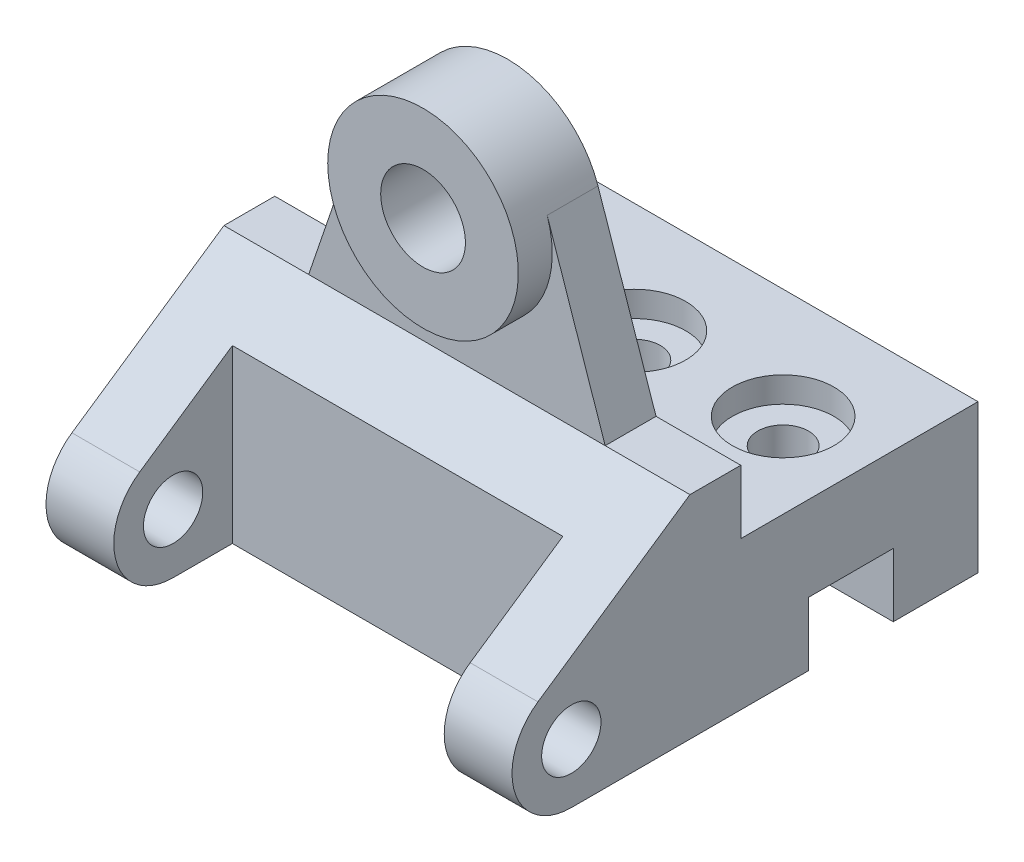
ISO-10303-21;
HEADER;
FILE_DESCRIPTION(('STEP AP214'),'2;1');
FILE_NAME('part.step','',(''),(''),'','','');
FILE_SCHEMA(('AUTOMOTIVE_DESIGN { 1 0 10303 214 1 1 1 1 }'));
ENDSEC;
DATA;
#1=APPLICATION_CONTEXT('core data for automotive mechanical design processes');
#2=APPLICATION_PROTOCOL_DEFINITION('international standard','automotive_design',2000,#1);
#3=PRODUCT_CONTEXT('',#1,'mechanical');
#4=PRODUCT('Part','Part','',(#3));
#5=PRODUCT_RELATED_PRODUCT_CATEGORY('part','',(#4));
#6=PRODUCT_DEFINITION_FORMATION('','',#4);
#7=PRODUCT_DEFINITION_CONTEXT('part definition',#1,'design');
#8=PRODUCT_DEFINITION('design','',#6,#7);
#9=PRODUCT_DEFINITION_SHAPE('','',#8);
#10=(LENGTH_UNIT() NAMED_UNIT(*) SI_UNIT(.MILLI.,.METRE.));
#11=(NAMED_UNIT(*) PLANE_ANGLE_UNIT() SI_UNIT($,.RADIAN.));
#12=(NAMED_UNIT(*) SI_UNIT($,.STERADIAN.) SOLID_ANGLE_UNIT());
#13=UNCERTAINTY_MEASURE_WITH_UNIT(LENGTH_MEASURE(1.E-05),#10,'distance_accuracy_value','');
#14=(GEOMETRIC_REPRESENTATION_CONTEXT(3) GLOBAL_UNCERTAINTY_ASSIGNED_CONTEXT((#13)) GLOBAL_UNIT_ASSIGNED_CONTEXT((#10,
#11,#12)) REPRESENTATION_CONTEXT('',''));
#15=CARTESIAN_POINT('',(0.,0.,0.));
#16=DIRECTION('',(0.,0.,1.));
#17=DIRECTION('',(1.,0.,0.));
#18=AXIS2_PLACEMENT_3D('',#15,#16,#17);
#19=CARTESIAN_POINT('',(55.,50.,28.));
#20=DIRECTION('',(0.,-1.,0.));
#21=DIRECTION('',(0.,0.,-1.));
#22=AXIS2_PLACEMENT_3D('',#19,#20,#21);
#23=PLANE('',#22);
#24=DIRECTION('',(0.,0.,-1.));
#25=VECTOR('',#24,1.);
#26=CARTESIAN_POINT('',(35.,50.,28.));
#27=LINE('',#26,#25);
#28=CARTESIAN_POINT('',(35.,50.,28.));
#29=VERTEX_POINT('',#28);
#30=CARTESIAN_POINT('',(35.,50.,16.));
#31=VERTEX_POINT('',#30);
#32=EDGE_CURVE('E224',#29,#31,#27,.T.);
#33=ORIENTED_EDGE('',*,*,#32,.F.);
#34=DIRECTION('',(-1.,0.,0.));
#35=VECTOR('',#34,1.);
#36=CARTESIAN_POINT('',(55.,50.,28.));
#37=LINE('',#36,#35);
#38=CARTESIAN_POINT('',(55.,50.,28.));
#39=VERTEX_POINT('',#38);
#40=EDGE_CURVE('E401',#39,#29,#37,.T.);
#41=ORIENTED_EDGE('',*,*,#40,.F.);
#42=DIRECTION('',(0.,0.,1.));
#43=VECTOR('',#42,1.);
#44=CARTESIAN_POINT('',(55.,50.,28.));
#45=LINE('',#44,#43);
#46=CARTESIAN_POINT('',(55.,50.,16.));
#47=VERTEX_POINT('',#46);
#48=EDGE_CURVE('E269',#47,#39,#45,.T.);
#49=ORIENTED_EDGE('',*,*,#48,.F.);
#50=DIRECTION('',(-1.,0.,0.));
#51=VECTOR('',#50,1.);
#52=CARTESIAN_POINT('',(55.,50.,16.));
#53=LINE('',#52,#51);
#54=EDGE_CURVE('E408',#47,#31,#53,.T.);
#55=ORIENTED_EDGE('',*,*,#54,.T.);
#56=EDGE_LOOP('',(#33,#41,#49,#55));
#57=FACE_BOUND('',#56,.T.);
#58=ADVANCED_FACE('F43',(#57),#23,.F.);
#59=CARTESIAN_POINT('',(55.,25.5724937407409,63.8789205238098));
#60=DIRECTION('',(0.,-0.826606695767211,-0.562780037414986));
#61=DIRECTION('',(0.,0.562780037414986,-0.826606695767211));
#62=AXIS2_PLACEMENT_3D('',#59,#60,#61);
#63=PLANE('',#62);
#64=DIRECTION('',(0.,-0.562780037414986,0.826606695767211));
#65=VECTOR('',#64,1.);
#66=CARTESIAN_POINT('',(-39.,25.5724937407409,63.8789205238098));
#67=LINE('',#66,#65);
#68=CARTESIAN_POINT('',(-39.,40.4683562761405,42.));
#69=VERTEX_POINT('',#68);
#70=CARTESIAN_POINT('',(-39.,25.5724937407409,63.8789205238098));
#71=VERTEX_POINT('',#70);
#72=EDGE_CURVE('E251',#69,#71,#67,.T.);
#73=ORIENTED_EDGE('',*,*,#72,.F.);
#74=DIRECTION('',(1.,0.,0.));
#75=VECTOR('',#74,1.);
#76=CARTESIAN_POINT('',(-39.,40.4683562761405,42.));
#77=LINE('',#76,#75);
#78=CARTESIAN_POINT('',(39.,40.4683562761405,42.));
#79=VERTEX_POINT('',#78);
#80=EDGE_CURVE('E238',#69,#79,#77,.T.);
#81=ORIENTED_EDGE('',*,*,#80,.T.);
#82=DIRECTION('',(0.,-0.562780037414986,0.826606695767211));
#83=VECTOR('',#82,1.);
#84=CARTESIAN_POINT('',(39.,25.5724937407409,63.8789205238098));
#85=LINE('',#84,#83);
#86=CARTESIAN_POINT('',(39.,25.5724937407409,63.8789205238098));
#87=VERTEX_POINT('',#86);
#88=EDGE_CURVE('E246',#79,#87,#85,.T.);
#89=ORIENTED_EDGE('',*,*,#88,.T.);
#90=DIRECTION('',(-1.,0.,0.));
#91=VECTOR('',#90,1.);
#92=CARTESIAN_POINT('',(55.,25.5724937407409,63.8789205238098));
#93=LINE('',#92,#91);
#94=CARTESIAN_POINT('',(55.,25.5724937407409,63.8789205238098));
#95=VERTEX_POINT('',#94);
#96=EDGE_CURVE('E412',#95,#87,#93,.T.);
#97=ORIENTED_EDGE('',*,*,#96,.F.);
#98=DIRECTION('',(0.,-0.562780037414986,0.826606695767211));
#99=VECTOR('',#98,1.);
#100=CARTESIAN_POINT('',(55.,25.5724937407409,63.8789205238098));
#101=LINE('',#100,#99);
#102=EDGE_CURVE('E275',#39,#95,#101,.T.);
#103=ORIENTED_EDGE('',*,*,#102,.F.);
#104=ORIENTED_EDGE('',*,*,#40,.T.);
#105=DIRECTION('',(1.,0.,0.));
#106=VECTOR('',#105,1.);
#107=CARTESIAN_POINT('',(0.,50.,28.));
#108=LINE('',#107,#106);
#109=CARTESIAN_POINT('',(-35.,50.,28.));
#110=VERTEX_POINT('',#109);
#111=EDGE_CURVE('E214',#110,#29,#108,.T.);
#112=ORIENTED_EDGE('',*,*,#111,.F.);
#113=CARTESIAN_POINT('',(-55.,50.,28.));
#114=VERTEX_POINT('',#113);
#115=EDGE_CURVE('E411',#110,#114,#37,.T.);
#116=ORIENTED_EDGE('',*,*,#115,.T.);
#117=DIRECTION('',(0.,-0.562780037414986,0.826606695767211));
#118=VECTOR('',#117,1.);
#119=CARTESIAN_POINT('',(-55.,25.5724937407409,63.8789205238098));
#120=LINE('',#119,#118);
#121=CARTESIAN_POINT('',(-55.,25.5724937407409,63.8789205238098));
#122=VERTEX_POINT('',#121);
#123=EDGE_CURVE('E298',#114,#122,#120,.T.);
#124=ORIENTED_EDGE('',*,*,#123,.T.);
#125=EDGE_CURVE('E438',#71,#122,#93,.T.);
#126=ORIENTED_EDGE('',*,*,#125,.F.);
#127=EDGE_LOOP('',(#73,#81,#89,#97,#103,#104,#112,#116,#124,#126));
#128=FACE_BOUND('',#127,.T.);
#129=ADVANCED_FACE('F409',(#128),#63,.F.);
#130=CARTESIAN_POINT('',(55.,14.,56.));
#131=DIRECTION('',(-1.,0.,0.));
#132=DIRECTION('',(0.,0.,1.));
#133=AXIS2_PLACEMENT_3D('',#130,#131,#132);
#134=CYLINDRICAL_SURFACE('',#133,14.);
#135=CARTESIAN_POINT('',(-39.,14.,56.));
#136=DIRECTION('',(1.,0.,0.));
#137=DIRECTION('',(0.,0.,-1.));
#138=AXIS2_PLACEMENT_3D('',#135,#136,#137);
#139=CIRCLE('',#138,14.);
#140=CARTESIAN_POINT('',(-39.,0.,56.));
#141=VERTEX_POINT('',#140);
#142=EDGE_CURVE('E253',#71,#141,#139,.T.);
#143=ORIENTED_EDGE('',*,*,#142,.F.);
#144=ORIENTED_EDGE('',*,*,#125,.T.);
#145=CARTESIAN_POINT('',(-55.,14.,56.));
#146=DIRECTION('',(1.,0.,0.));
#147=DIRECTION('',(0.,0.,1.));
#148=AXIS2_PLACEMENT_3D('',#145,#146,#147);
#149=CIRCLE('',#148,14.);
#150=CARTESIAN_POINT('',(-55.,0.,56.));
#151=VERTEX_POINT('',#150);
#152=EDGE_CURVE('E297',#122,#151,#149,.T.);
#153=ORIENTED_EDGE('',*,*,#152,.T.);
#154=DIRECTION('',(-1.,0.,0.));
#155=VECTOR('',#154,1.);
#156=CARTESIAN_POINT('',(55.,0.,56.));
#157=LINE('',#156,#155);
#158=EDGE_CURVE('E439',#141,#151,#157,.T.);
#159=ORIENTED_EDGE('',*,*,#158,.F.);
#160=EDGE_LOOP('',(#143,#144,#153,#159));
#161=FACE_BOUND('',#160,.T.);
#162=ADVANCED_FACE('F437',(#161),#134,.T.);
#163=CARTESIAN_POINT('',(55.,14.,56.));
#164=DIRECTION('',(-1.,0.,0.));
#165=DIRECTION('',(0.,0.,1.));
#166=AXIS2_PLACEMENT_3D('',#163,#164,#165);
#167=CYLINDRICAL_SURFACE('',#166,7.);
#168=CARTESIAN_POINT('',(-55.,14.,56.));
#169=DIRECTION('',(1.,0.,0.));
#170=DIRECTION('',(0.,0.,-1.));
#171=AXIS2_PLACEMENT_3D('',#168,#169,#170);
#172=CIRCLE('',#171,7.);
#173=CARTESIAN_POINT('',(-55.,14.,49.));
#174=VERTEX_POINT('',#173);
#175=EDGE_CURVE('E254',#174,#174,#172,.T.);
#176=ORIENTED_EDGE('',*,*,#175,.F.);
#177=EDGE_LOOP('',(#176));
#178=FACE_BOUND('',#177,.T.);
#179=CARTESIAN_POINT('',(-39.,14.,56.));
#180=DIRECTION('',(1.,0.,0.));
#181=DIRECTION('',(0.,0.,-1.));
#182=AXIS2_PLACEMENT_3D('',#179,#180,#181);
#183=CIRCLE('',#182,7.);
#184=CARTESIAN_POINT('',(-39.,14.,49.));
#185=VERTEX_POINT('',#184);
#186=EDGE_CURVE('E247',#185,#185,#183,.T.);
#187=ORIENTED_EDGE('',*,*,#186,.T.);
#188=EDGE_LOOP('',(#187));
#189=FACE_BOUND('',#188,.T.);
#190=ADVANCED_FACE('F422',(#178,#189),#167,.F.);
#191=CARTESIAN_POINT('',(55.,14.,56.));
#192=DIRECTION('',(-1.,0.,0.));
#193=DIRECTION('',(0.,0.,1.));
#194=AXIS2_PLACEMENT_3D('',#191,#192,#193);
#195=PLANE('',#194);
#196=DIRECTION('',(0.,1.,0.));
#197=VECTOR('',#196,1.);
#198=CARTESIAN_POINT('',(55.,35.,-40.));
#199=LINE('',#198,#197);
#200=CARTESIAN_POINT('',(55.,0.,-40.));
#201=VERTEX_POINT('',#200);
#202=CARTESIAN_POINT('',(55.,35.,-40.));
#203=VERTEX_POINT('',#202);
#204=EDGE_CURVE('E265',#201,#203,#199,.T.);
#205=ORIENTED_EDGE('',*,*,#204,.T.);
#206=DIRECTION('',(0.,0.,1.));
#207=VECTOR('',#206,1.);
#208=CARTESIAN_POINT('',(55.,35.,16.));
#209=LINE('',#208,#207);
#210=CARTESIAN_POINT('',(55.,35.,16.));
#211=VERTEX_POINT('',#210);
#212=EDGE_CURVE('E264',#203,#211,#209,.T.);
#213=ORIENTED_EDGE('',*,*,#212,.T.);
#214=DIRECTION('',(0.,1.,0.));
#215=VECTOR('',#214,1.);
#216=CARTESIAN_POINT('',(55.,50.,16.));
#217=LINE('',#216,#215);
#218=EDGE_CURVE('E268',#211,#47,#217,.T.);
#219=ORIENTED_EDGE('',*,*,#218,.T.);
#220=ORIENTED_EDGE('',*,*,#48,.T.);
#221=ORIENTED_EDGE('',*,*,#102,.T.);
#222=CARTESIAN_POINT('',(55.,14.,56.));
#223=DIRECTION('',(1.,0.,0.));
#224=DIRECTION('',(0.,0.,1.));
#225=AXIS2_PLACEMENT_3D('',#222,#223,#224);
#226=CIRCLE('',#225,14.);
#227=CARTESIAN_POINT('',(55.,0.,56.));
#228=VERTEX_POINT('',#227);
#229=EDGE_CURVE('E273',#95,#228,#226,.T.);
#230=ORIENTED_EDGE('',*,*,#229,.T.);
#231=DIRECTION('',(0.,0.,-1.));
#232=VECTOR('',#231,1.);
#233=CARTESIAN_POINT('',(55.,0.,0.));
#234=LINE('',#233,#232);
#235=CARTESIAN_POINT('',(55.,0.,0.));
#236=VERTEX_POINT('',#235);
#237=EDGE_CURVE('E277',#228,#236,#234,.T.);
#238=ORIENTED_EDGE('',*,*,#237,.T.);
#239=DIRECTION('',(0.,1.,0.));
#240=VECTOR('',#239,1.);
#241=CARTESIAN_POINT('',(55.,0.,0.));
#242=LINE('',#241,#240);
#243=CARTESIAN_POINT('',(55.,15.,0.));
#244=VERTEX_POINT('',#243);
#245=EDGE_CURVE('E279',#236,#244,#242,.T.);
#246=ORIENTED_EDGE('',*,*,#245,.T.);
#247=DIRECTION('',(0.,0.,-1.));
#248=VECTOR('',#247,1.);
#249=CARTESIAN_POINT('',(55.,15.,0.));
#250=LINE('',#249,#248);
#251=CARTESIAN_POINT('',(55.,15.,-20.));
#252=VERTEX_POINT('',#251);
#253=EDGE_CURVE('E278',#244,#252,#250,.T.);
#254=ORIENTED_EDGE('',*,*,#253,.T.);
#255=DIRECTION('',(0.,-1.,0.));
#256=VECTOR('',#255,1.);
#257=CARTESIAN_POINT('',(55.,0.,-20.));
#258=LINE('',#257,#256);
#259=CARTESIAN_POINT('',(55.,0.,-20.));
#260=VERTEX_POINT('',#259);
#261=EDGE_CURVE('E285',#252,#260,#258,.T.);
#262=ORIENTED_EDGE('',*,*,#261,.T.);
#263=DIRECTION('',(0.,0.,-1.));
#264=VECTOR('',#263,1.);
#265=CARTESIAN_POINT('',(55.,0.,-40.));
#266=LINE('',#265,#264);
#267=EDGE_CURVE('E282',#260,#201,#266,.T.);
#268=ORIENTED_EDGE('',*,*,#267,.T.);
#269=EDGE_LOOP('',(#205,#213,#219,#220,#221,#230,#238,#246,#254,#262,#268));
#270=FACE_BOUND('',#269,.T.);
#271=CARTESIAN_POINT('',(55.,14.,56.));
#272=DIRECTION('',(1.,0.,0.));
#273=DIRECTION('',(0.,0.,-1.));
#274=AXIS2_PLACEMENT_3D('',#271,#272,#273);
#275=CIRCLE('',#274,7.);
#276=CARTESIAN_POINT('',(55.,14.,49.));
#277=VERTEX_POINT('',#276);
#278=EDGE_CURVE('E258',#277,#277,#275,.T.);
#279=ORIENTED_EDGE('',*,*,#278,.F.);
#280=EDGE_LOOP('',(#279));
#281=FACE_BOUND('',#280,.T.);
#282=ADVANCED_FACE('F359',(#270,#281),#195,.F.);
#283=CARTESIAN_POINT('',(-55.,14.,56.));
#284=DIRECTION('',(-1.,0.,0.));
#285=DIRECTION('',(0.,0.,1.));
#286=AXIS2_PLACEMENT_3D('',#283,#284,#285);
#287=PLANE('',#286);
#288=DIRECTION('',(0.,1.,0.));
#289=VECTOR('',#288,1.);
#290=CARTESIAN_POINT('',(-55.,35.,-40.));
#291=LINE('',#290,#289);
#292=CARTESIAN_POINT('',(-55.,0.,-40.));
#293=VERTEX_POINT('',#292);
#294=CARTESIAN_POINT('',(-55.,35.,-40.));
#295=VERTEX_POINT('',#294);
#296=EDGE_CURVE('E259',#293,#295,#291,.T.);
#297=ORIENTED_EDGE('',*,*,#296,.F.);
#298=DIRECTION('',(0.,0.,-1.));
#299=VECTOR('',#298,1.);
#300=CARTESIAN_POINT('',(-55.,0.,-40.));
#301=LINE('',#300,#299);
#302=CARTESIAN_POINT('',(-55.,0.,-20.));
#303=VERTEX_POINT('',#302);
#304=EDGE_CURVE('E266',#303,#293,#301,.T.);
#305=ORIENTED_EDGE('',*,*,#304,.F.);
#306=DIRECTION('',(0.,-1.,0.));
#307=VECTOR('',#306,1.);
#308=CARTESIAN_POINT('',(-55.,0.,-20.));
#309=LINE('',#308,#307);
#310=CARTESIAN_POINT('',(-55.,15.,-20.));
#311=VERTEX_POINT('',#310);
#312=EDGE_CURVE('E310',#311,#303,#309,.T.);
#313=ORIENTED_EDGE('',*,*,#312,.F.);
#314=DIRECTION('',(0.,0.,-1.));
#315=VECTOR('',#314,1.);
#316=CARTESIAN_POINT('',(-55.,15.,0.));
#317=LINE('',#316,#315);
#318=CARTESIAN_POINT('',(-55.,15.,0.));
#319=VERTEX_POINT('',#318);
#320=EDGE_CURVE('E308',#319,#311,#317,.T.);
#321=ORIENTED_EDGE('',*,*,#320,.F.);
#322=DIRECTION('',(0.,1.,0.));
#323=VECTOR('',#322,1.);
#324=CARTESIAN_POINT('',(-55.,0.,0.));
#325=LINE('',#324,#323);
#326=CARTESIAN_POINT('',(-55.,0.,0.));
#327=VERTEX_POINT('',#326);
#328=EDGE_CURVE('E303',#327,#319,#325,.T.);
#329=ORIENTED_EDGE('',*,*,#328,.F.);
#330=DIRECTION('',(0.,0.,-1.));
#331=VECTOR('',#330,1.);
#332=CARTESIAN_POINT('',(-55.,0.,0.));
#333=LINE('',#332,#331);
#334=EDGE_CURVE('E301',#151,#327,#333,.T.);
#335=ORIENTED_EDGE('',*,*,#334,.F.);
#336=ORIENTED_EDGE('',*,*,#152,.F.);
#337=ORIENTED_EDGE('',*,*,#123,.F.);
#338=DIRECTION('',(0.,0.,1.));
#339=VECTOR('',#338,1.);
#340=CARTESIAN_POINT('',(-55.,50.,28.));
#341=LINE('',#340,#339);
#342=CARTESIAN_POINT('',(-55.,50.,16.));
#343=VERTEX_POINT('',#342);
#344=EDGE_CURVE('E291',#343,#114,#341,.T.);
#345=ORIENTED_EDGE('',*,*,#344,.F.);
#346=DIRECTION('',(0.,1.,0.));
#347=VECTOR('',#346,1.);
#348=CARTESIAN_POINT('',(-55.,50.,16.));
#349=LINE('',#348,#347);
#350=CARTESIAN_POINT('',(-55.,35.,16.));
#351=VERTEX_POINT('',#350);
#352=EDGE_CURVE('E292',#351,#343,#349,.T.);
#353=ORIENTED_EDGE('',*,*,#352,.F.);
#354=DIRECTION('',(0.,0.,1.));
#355=VECTOR('',#354,1.);
#356=CARTESIAN_POINT('',(-55.,35.,16.));
#357=LINE('',#356,#355);
#358=EDGE_CURVE('E288',#295,#351,#357,.T.);
#359=ORIENTED_EDGE('',*,*,#358,.F.);
#360=EDGE_LOOP('',(#297,#305,#313,#321,#329,#335,#336,#337,#345,#353,#359));
#361=FACE_BOUND('',#360,.T.);
#362=ORIENTED_EDGE('',*,*,#175,.T.);
#363=EDGE_LOOP('',(#362));
#364=FACE_BOUND('',#363,.T.);
#365=ADVANCED_FACE('F347',(#361,#364),#287,.T.);
#366=CARTESIAN_POINT('',(55.,35.,-40.));
#367=DIRECTION('',(0.,0.,1.));
#368=DIRECTION('',(0.,-1.,0.));
#369=AXIS2_PLACEMENT_3D('',#366,#367,#368);
#370=PLANE('',#369);
#371=ORIENTED_EDGE('',*,*,#296,.T.);
#372=DIRECTION('',(-1.,0.,0.));
#373=VECTOR('',#372,1.);
#374=CARTESIAN_POINT('',(55.,35.,-40.));
#375=LINE('',#374,#373);
#376=EDGE_CURVE('E12',#203,#295,#375,.T.);
#377=ORIENTED_EDGE('',*,*,#376,.F.);
#378=ORIENTED_EDGE('',*,*,#204,.F.);
#379=DIRECTION('',(-1.,0.,0.));
#380=VECTOR('',#379,1.);
#381=CARTESIAN_POINT('',(55.,0.,-40.));
#382=LINE('',#381,#380);
#383=EDGE_CURVE('E289',#201,#293,#382,.T.);
#384=ORIENTED_EDGE('',*,*,#383,.T.);
#385=EDGE_LOOP('',(#371,#377,#378,#384));
#386=FACE_BOUND('',#385,.T.);
#387=ADVANCED_FACE('F44',(#386),#370,.F.);
#388=CARTESIAN_POINT('',(55.,35.,16.));
#389=DIRECTION('',(0.,-1.,0.));
#390=DIRECTION('',(0.,0.,-1.));
#391=AXIS2_PLACEMENT_3D('',#388,#389,#390);
#392=PLANE('',#391);
#393=CARTESIAN_POINT('',(35.,35.,-14.));
#394=DIRECTION('',(0.,1.,0.));
#395=DIRECTION('',(0.,0.,1.));
#396=AXIS2_PLACEMENT_3D('',#393,#394,#395);
#397=CIRCLE('',#396,12.);
#398=CARTESIAN_POINT('',(35.,35.,-1.99999999999999));
#399=VERTEX_POINT('',#398);
#400=EDGE_CURVE('E575',#399,#399,#397,.T.);
#401=ORIENTED_EDGE('',*,*,#400,.F.);
#402=EDGE_LOOP('',(#401));
#403=FACE_BOUND('',#402,.T.);
#404=CARTESIAN_POINT('',(0.,35.,-14.));
#405=DIRECTION('',(0.,1.,0.));
#406=DIRECTION('',(0.,0.,1.));
#407=AXIS2_PLACEMENT_3D('',#404,#405,#406);
#408=CIRCLE('',#407,12.);
#409=CARTESIAN_POINT('',(0.,35.,-1.99999999999999));
#410=VERTEX_POINT('',#409);
#411=EDGE_CURVE('E583',#410,#410,#408,.T.);
#412=ORIENTED_EDGE('',*,*,#411,.F.);
#413=EDGE_LOOP('',(#412));
#414=FACE_BOUND('',#413,.T.);
#415=CARTESIAN_POINT('',(-35.,35.,-14.));
#416=DIRECTION('',(0.,1.,0.));
#417=DIRECTION('',(0.,0.,1.));
#418=AXIS2_PLACEMENT_3D('',#415,#416,#417);
#419=CIRCLE('',#418,12.);
#420=CARTESIAN_POINT('',(-35.,35.,-1.99999999999999));
#421=VERTEX_POINT('',#420);
#422=EDGE_CURVE('E365',#421,#421,#419,.T.);
#423=ORIENTED_EDGE('',*,*,#422,.F.);
#424=EDGE_LOOP('',(#423));
#425=FACE_BOUND('',#424,.T.);
#426=ORIENTED_EDGE('',*,*,#358,.T.);
#427=DIRECTION('',(-1.,0.,0.));
#428=VECTOR('',#427,1.);
#429=CARTESIAN_POINT('',(55.,35.,16.));
#430=LINE('',#429,#428);
#431=EDGE_CURVE('E52',#211,#351,#430,.T.);
#432=ORIENTED_EDGE('',*,*,#431,.F.);
#433=ORIENTED_EDGE('',*,*,#212,.F.);
#434=ORIENTED_EDGE('',*,*,#376,.T.);
#435=EDGE_LOOP('',(#426,#432,#433,#434));
#436=FACE_BOUND('',#435,.T.);
#437=ADVANCED_FACE('F481',(#403,#414,#425,#436),#392,.F.);
#438=CARTESIAN_POINT('',(55.,50.,16.));
#439=DIRECTION('',(0.,0.,1.));
#440=DIRECTION('',(0.,-1.,0.));
#441=AXIS2_PLACEMENT_3D('',#438,#439,#440);
#442=PLANE('',#441);
#443=ORIENTED_EDGE('',*,*,#352,.T.);
#444=CARTESIAN_POINT('',(-35.,50.,16.));
#445=VERTEX_POINT('',#444);
#446=EDGE_CURVE('E211',#445,#343,#53,.T.);
#447=ORIENTED_EDGE('',*,*,#446,.F.);
#448=DIRECTION('',(-0.322220189663275,-0.946664750253945,0.));
#449=VECTOR('',#448,1.);
#450=CARTESIAN_POINT('',(-46.6178199967859,15.8674998694345,16.));
#451=LINE('',#450,#449);
#452=CARTESIAN_POINT('',(-21.2999568807138,90.2499542674237,16.));
#453=VERTEX_POINT('',#452);
#454=EDGE_CURVE('E205',#453,#445,#451,.T.);
#455=ORIENTED_EDGE('',*,*,#454,.F.);
#456=CARTESIAN_POINT('',(0.,83.,16.));
#457=DIRECTION('',(0.,0.,-1.));
#458=DIRECTION('',(-1.,0.,0.));
#459=AXIS2_PLACEMENT_3D('',#456,#457,#458);
#460=CIRCLE('',#459,22.5);
#461=CARTESIAN_POINT('',(21.2999568807138,90.2499542674237,16.));
#462=VERTEX_POINT('',#461);
#463=EDGE_CURVE('E184',#453,#462,#460,.T.);
#464=ORIENTED_EDGE('',*,*,#463,.T.);
#465=DIRECTION('',(0.322220189663275,-0.946664750253945,0.));
#466=VECTOR('',#465,1.);
#467=CARTESIAN_POINT('',(46.6178199967858,15.8674998694345,16.));
#468=LINE('',#467,#466);
#469=EDGE_CURVE('E215',#462,#31,#468,.T.);
#470=ORIENTED_EDGE('',*,*,#469,.T.);
#471=ORIENTED_EDGE('',*,*,#54,.F.);
#472=ORIENTED_EDGE('',*,*,#218,.F.);
#473=ORIENTED_EDGE('',*,*,#431,.T.);
#474=EDGE_LOOP('',(#443,#447,#455,#464,#470,#471,#472,#473));
#475=FACE_BOUND('',#474,.T.);
#476=CARTESIAN_POINT('',(0.,83.,16.));
#477=DIRECTION('',(0.,0.,-1.));
#478=DIRECTION('',(-1.,0.,0.));
#479=AXIS2_PLACEMENT_3D('',#476,#477,#478);
#480=CIRCLE('',#479,10.);
#481=CARTESIAN_POINT('',(-10.,83.,16.));
#482=VERTEX_POINT('',#481);
#483=EDGE_CURVE('E198',#482,#482,#480,.T.);
#484=ORIENTED_EDGE('',*,*,#483,.F.);
#485=EDGE_LOOP('',(#484));
#486=FACE_BOUND('',#485,.T.);
#487=ADVANCED_FACE('F207',(#475,#486),#442,.F.);
#488=ORIENTED_EDGE('',*,*,#115,.F.);
#489=DIRECTION('',(0.,0.,-1.));
#490=VECTOR('',#489,1.);
#491=CARTESIAN_POINT('',(-35.,50.,28.));
#492=LINE('',#491,#490);
#493=EDGE_CURVE('E202',#110,#445,#492,.T.);
#494=ORIENTED_EDGE('',*,*,#493,.T.);
#495=ORIENTED_EDGE('',*,*,#446,.T.);
#496=ORIENTED_EDGE('',*,*,#344,.T.);
#497=EDGE_LOOP('',(#488,#494,#495,#496));
#498=FACE_BOUND('',#497,.T.);
#499=ADVANCED_FACE('F472',(#498),#23,.F.);
#500=ORIENTED_EDGE('',*,*,#96,.T.);
#501=CARTESIAN_POINT('',(39.,14.,56.));
#502=DIRECTION('',(1.,0.,0.));
#503=DIRECTION('',(0.,0.,-1.));
#504=AXIS2_PLACEMENT_3D('',#501,#502,#503);
#505=CIRCLE('',#504,14.);
#506=CARTESIAN_POINT('',(39.,0.,56.));
#507=VERTEX_POINT('',#506);
#508=EDGE_CURVE('E244',#87,#507,#505,.T.);
#509=ORIENTED_EDGE('',*,*,#508,.T.);
#510=EDGE_CURVE('E444',#228,#507,#157,.T.);
#511=ORIENTED_EDGE('',*,*,#510,.F.);
#512=ORIENTED_EDGE('',*,*,#229,.F.);
#513=EDGE_LOOP('',(#500,#509,#511,#512));
#514=FACE_BOUND('',#513,.T.);
#515=ADVANCED_FACE('F464',(#514),#134,.T.);
#516=CARTESIAN_POINT('',(55.,0.,0.));
#517=DIRECTION('',(0.,1.,0.));
#518=DIRECTION('',(0.,0.,1.));
#519=AXIS2_PLACEMENT_3D('',#516,#517,#518);
#520=PLANE('',#519);
#521=ORIENTED_EDGE('',*,*,#510,.T.);
#522=DIRECTION('',(0.,0.,-1.));
#523=VECTOR('',#522,1.);
#524=CARTESIAN_POINT('',(39.,0.,70.));
#525=LINE('',#524,#523);
#526=CARTESIAN_POINT('',(39.,0.,42.));
#527=VERTEX_POINT('',#526);
#528=EDGE_CURVE('E223',#507,#527,#525,.T.);
#529=ORIENTED_EDGE('',*,*,#528,.T.);
#530=DIRECTION('',(1.,0.,0.));
#531=VECTOR('',#530,1.);
#532=CARTESIAN_POINT('',(-39.,0.,42.));
#533=LINE('',#532,#531);
#534=CARTESIAN_POINT('',(-39.,0.,42.));
#535=VERTEX_POINT('',#534);
#536=EDGE_CURVE('E232',#535,#527,#533,.T.);
#537=ORIENTED_EDGE('',*,*,#536,.F.);
#538=DIRECTION('',(0.,0.,-1.));
#539=VECTOR('',#538,1.);
#540=CARTESIAN_POINT('',(-39.,0.,70.));
#541=LINE('',#540,#539);
#542=EDGE_CURVE('E226',#141,#535,#541,.T.);
#543=ORIENTED_EDGE('',*,*,#542,.F.);
#544=ORIENTED_EDGE('',*,*,#158,.T.);
#545=ORIENTED_EDGE('',*,*,#334,.T.);
#546=DIRECTION('',(-1.,0.,0.));
#547=VECTOR('',#546,1.);
#548=CARTESIAN_POINT('',(55.,0.,0.));
#549=LINE('',#548,#547);
#550=EDGE_CURVE('E447',#236,#327,#549,.T.);
#551=ORIENTED_EDGE('',*,*,#550,.F.);
#552=ORIENTED_EDGE('',*,*,#237,.F.);
#553=EDGE_LOOP('',(#521,#529,#537,#543,#544,#545,#551,#552));
#554=FACE_BOUND('',#553,.T.);
#555=ADVANCED_FACE('F457',(#554),#520,.F.);
#556=CARTESIAN_POINT('',(55.,0.,0.));
#557=DIRECTION('',(0.,0.,1.));
#558=DIRECTION('',(0.,-1.,0.));
#559=AXIS2_PLACEMENT_3D('',#556,#557,#558);
#560=PLANE('',#559);
#561=ORIENTED_EDGE('',*,*,#328,.T.);
#562=DIRECTION('',(-1.,0.,0.));
#563=VECTOR('',#562,1.);
#564=CARTESIAN_POINT('',(55.,15.,0.));
#565=LINE('',#564,#563);
#566=EDGE_CURVE('E317',#244,#319,#565,.T.);
#567=ORIENTED_EDGE('',*,*,#566,.F.);
#568=ORIENTED_EDGE('',*,*,#245,.F.);
#569=ORIENTED_EDGE('',*,*,#550,.T.);
#570=EDGE_LOOP('',(#561,#567,#568,#569));
#571=FACE_BOUND('',#570,.T.);
#572=ADVANCED_FACE('F453',(#571),#560,.F.);
#573=CARTESIAN_POINT('',(55.,15.,0.));
#574=DIRECTION('',(0.,1.,0.));
#575=DIRECTION('',(0.,0.,1.));
#576=AXIS2_PLACEMENT_3D('',#573,#574,#575);
#577=PLANE('',#576);
#578=DIRECTION('',(-1.,0.,0.));
#579=VECTOR('',#578,1.);
#580=CARTESIAN_POINT('',(55.,15.,-20.));
#581=LINE('',#580,#579);
#582=CARTESIAN_POINT('',(35.,14.9995,-20.));
#583=VERTEX_POINT('',#582);
#584=CARTESIAN_POINT('',(0.,14.9995,-20.));
#585=VERTEX_POINT('',#584);
#586=EDGE_CURVE('E50',#583,#585,#581,.T.);
#587=ORIENTED_EDGE('',*,*,#586,.F.);
#588=CARTESIAN_POINT('',(35.,15.,-14.));
#589=DIRECTION('',(0.,1.,0.));
#590=DIRECTION('',(0.,0.,1.));
#591=AXIS2_PLACEMENT_3D('',#588,#589,#590);
#592=CIRCLE('',#591,6.00000000000001);
#593=EDGE_CURVE('E56',#583,#583,#592,.T.);
#594=ORIENTED_EDGE('',*,*,#593,.T.);
#595=EDGE_CURVE('E322',#252,#583,#581,.T.);
#596=ORIENTED_EDGE('',*,*,#595,.F.);
#597=ORIENTED_EDGE('',*,*,#253,.F.);
#598=ORIENTED_EDGE('',*,*,#566,.T.);
#599=ORIENTED_EDGE('',*,*,#320,.T.);
#600=CARTESIAN_POINT('',(-35.,14.9995,-20.));
#601=VERTEX_POINT('',#600);
#602=EDGE_CURVE('E316',#601,#311,#581,.T.);
#603=ORIENTED_EDGE('',*,*,#602,.F.);
#604=CARTESIAN_POINT('',(-35.,15.,-14.));
#605=DIRECTION('',(0.,1.,0.));
#606=DIRECTION('',(0.,0.,1.));
#607=AXIS2_PLACEMENT_3D('',#604,#605,#606);
#608=CIRCLE('',#607,6.00000000000001);
#609=EDGE_CURVE('E385',#601,#601,#608,.T.);
#610=ORIENTED_EDGE('',*,*,#609,.T.);
#611=EDGE_CURVE('E327',#585,#601,#581,.T.);
#612=ORIENTED_EDGE('',*,*,#611,.F.);
#613=CARTESIAN_POINT('',(0.,15.,-14.));
#614=DIRECTION('',(0.,1.,0.));
#615=DIRECTION('',(0.,0.,1.));
#616=AXIS2_PLACEMENT_3D('',#613,#614,#615);
#617=CIRCLE('',#616,6.00000000000001);
#618=EDGE_CURVE('E362',#585,#585,#617,.T.);
#619=ORIENTED_EDGE('',*,*,#618,.T.);
#620=EDGE_LOOP('',(#587,#594,#596,#597,#598,#599,#603,#610,#612,#619));
#621=FACE_BOUND('',#620,.T.);
#622=ADVANCED_FACE('F337',(#621),#577,.F.);
#623=CARTESIAN_POINT('',(55.,0.,-20.));
#624=DIRECTION('',(0.,0.,-1.));
#625=DIRECTION('',(0.,1.,0.));
#626=AXIS2_PLACEMENT_3D('',#623,#624,#625);
#627=PLANE('',#626);
#628=ORIENTED_EDGE('',*,*,#595,.T.);
#629=ORIENTED_EDGE('',*,*,#586,.T.);
#630=ORIENTED_EDGE('',*,*,#611,.T.);
#631=ORIENTED_EDGE('',*,*,#602,.T.);
#632=ORIENTED_EDGE('',*,*,#312,.T.);
#633=DIRECTION('',(-1.,0.,0.));
#634=VECTOR('',#633,1.);
#635=CARTESIAN_POINT('',(55.,0.,-20.));
#636=LINE('',#635,#634);
#637=EDGE_CURVE('E314',#260,#303,#636,.T.);
#638=ORIENTED_EDGE('',*,*,#637,.F.);
#639=ORIENTED_EDGE('',*,*,#261,.F.);
#640=EDGE_LOOP('',(#628,#629,#630,#631,#632,#638,#639));
#641=FACE_BOUND('',#640,.T.);
#642=ADVANCED_FACE('F335',(#641),#627,.F.);
#643=CARTESIAN_POINT('',(55.,0.,-40.));
#644=DIRECTION('',(0.,1.,0.));
#645=DIRECTION('',(0.,0.,1.));
#646=AXIS2_PLACEMENT_3D('',#643,#644,#645);
#647=PLANE('',#646);
#648=ORIENTED_EDGE('',*,*,#304,.T.);
#649=ORIENTED_EDGE('',*,*,#383,.F.);
#650=ORIENTED_EDGE('',*,*,#267,.F.);
#651=ORIENTED_EDGE('',*,*,#637,.T.);
#652=EDGE_LOOP('',(#648,#649,#650,#651));
#653=FACE_BOUND('',#652,.T.);
#654=ADVANCED_FACE('F348',(#653),#647,.F.);
#655=CARTESIAN_POINT('',(39.,14.,56.));
#656=DIRECTION('',(1.,0.,0.));
#657=DIRECTION('',(0.,0.,-1.));
#658=AXIS2_PLACEMENT_3D('',#655,#656,#657);
#659=CIRCLE('',#658,7.);
#660=CARTESIAN_POINT('',(39.,14.,49.));
#661=VERTEX_POINT('',#660);
#662=EDGE_CURVE('E241',#661,#661,#659,.T.);
#663=ORIENTED_EDGE('',*,*,#662,.F.);
#664=EDGE_LOOP('',(#663));
#665=FACE_BOUND('',#664,.T.);
#666=ORIENTED_EDGE('',*,*,#278,.T.);
#667=EDGE_LOOP('',(#666));
#668=FACE_BOUND('',#667,.T.);
#669=ADVANCED_FACE('F431',(#665,#668),#167,.F.);
#670=CARTESIAN_POINT('',(-39.,0.,0.));
#671=DIRECTION('',(1.,0.,0.));
#672=DIRECTION('',(0.,0.,-1.));
#673=AXIS2_PLACEMENT_3D('',#670,#671,#672);
#674=PLANE('',#673);
#675=ORIENTED_EDGE('',*,*,#186,.F.);
#676=EDGE_LOOP('',(#675));
#677=FACE_BOUND('',#676,.T.);
#678=ORIENTED_EDGE('',*,*,#72,.T.);
#679=ORIENTED_EDGE('',*,*,#142,.T.);
#680=ORIENTED_EDGE('',*,*,#542,.T.);
#681=DIRECTION('',(0.,1.,0.));
#682=VECTOR('',#681,1.);
#683=CARTESIAN_POINT('',(-39.,40.4683562761405,42.));
#684=LINE('',#683,#682);
#685=EDGE_CURVE('E234',#535,#69,#684,.T.);
#686=ORIENTED_EDGE('',*,*,#685,.T.);
#687=EDGE_LOOP('',(#678,#679,#680,#686));
#688=FACE_BOUND('',#687,.T.);
#689=ADVANCED_FACE('F430',(#677,#688),#674,.T.);
#690=CARTESIAN_POINT('',(39.,0.,0.));
#691=DIRECTION('',(1.,0.,0.));
#692=DIRECTION('',(0.,0.,-1.));
#693=AXIS2_PLACEMENT_3D('',#690,#691,#692);
#694=PLANE('',#693);
#695=ORIENTED_EDGE('',*,*,#662,.T.);
#696=EDGE_LOOP('',(#695));
#697=FACE_BOUND('',#696,.T.);
#698=DIRECTION('',(0.,1.,0.));
#699=VECTOR('',#698,1.);
#700=CARTESIAN_POINT('',(39.,40.4683562761405,42.));
#701=LINE('',#700,#699);
#702=EDGE_CURVE('E231',#527,#79,#701,.T.);
#703=ORIENTED_EDGE('',*,*,#702,.F.);
#704=ORIENTED_EDGE('',*,*,#528,.F.);
#705=ORIENTED_EDGE('',*,*,#508,.F.);
#706=ORIENTED_EDGE('',*,*,#88,.F.);
#707=EDGE_LOOP('',(#703,#704,#705,#706));
#708=FACE_BOUND('',#707,.T.);
#709=ADVANCED_FACE('F429',(#697,#708),#694,.F.);
#710=CARTESIAN_POINT('',(-39.,40.4683562761405,42.));
#711=DIRECTION('',(0.,0.,-1.));
#712=DIRECTION('',(0.,1.,0.));
#713=AXIS2_PLACEMENT_3D('',#710,#711,#712);
#714=PLANE('',#713);
#715=ORIENTED_EDGE('',*,*,#702,.T.);
#716=ORIENTED_EDGE('',*,*,#80,.F.);
#717=ORIENTED_EDGE('',*,*,#685,.F.);
#718=ORIENTED_EDGE('',*,*,#536,.T.);
#719=EDGE_LOOP('',(#715,#716,#717,#718));
#720=FACE_BOUND('',#719,.T.);
#721=ADVANCED_FACE('F463',(#720),#714,.F.);
#722=CARTESIAN_POINT('',(46.6178199967858,15.8674998694345,28.));
#723=DIRECTION('',(0.946664750253945,0.322220189663275,0.));
#724=DIRECTION('',(-0.322220189663275,0.946664750253945,0.));
#725=AXIS2_PLACEMENT_3D('',#722,#723,#724);
#726=PLANE('',#725);
#727=ORIENTED_EDGE('',*,*,#469,.F.);
#728=DIRECTION('',(0.,0.,-1.));
#729=VECTOR('',#728,1.);
#730=CARTESIAN_POINT('',(21.2999568807138,90.2499542674236,28.));
#731=LINE('',#730,#729);
#732=CARTESIAN_POINT('',(21.2999568807138,90.2499542674237,28.));
#733=VERTEX_POINT('',#732);
#734=EDGE_CURVE('E189',#733,#462,#731,.T.);
#735=ORIENTED_EDGE('',*,*,#734,.F.);
#736=DIRECTION('',(0.322220189663275,-0.946664750253945,0.));
#737=VECTOR('',#736,1.);
#738=CARTESIAN_POINT('',(46.6178199967858,15.8674998694345,28.));
#739=LINE('',#738,#737);
#740=EDGE_CURVE('E219',#733,#29,#739,.T.);
#741=ORIENTED_EDGE('',*,*,#740,.T.);
#742=ORIENTED_EDGE('',*,*,#32,.T.);
#743=EDGE_LOOP('',(#727,#735,#741,#742));
#744=FACE_BOUND('',#743,.T.);
#745=ADVANCED_FACE('F396',(#744),#726,.T.);
#746=CARTESIAN_POINT('',(-46.6178199967859,15.8674998694345,28.));
#747=DIRECTION('',(0.946664750253944,-0.322220189663275,0.));
#748=DIRECTION('',(0.322220189663275,0.946664750253945,0.));
#749=AXIS2_PLACEMENT_3D('',#746,#747,#748);
#750=PLANE('',#749);
#751=ORIENTED_EDGE('',*,*,#454,.T.);
#752=ORIENTED_EDGE('',*,*,#493,.F.);
#753=DIRECTION('',(-0.322220189663275,-0.946664750253945,0.));
#754=VECTOR('',#753,1.);
#755=CARTESIAN_POINT('',(-46.6178199967859,15.8674998694345,28.));
#756=LINE('',#755,#754);
#757=CARTESIAN_POINT('',(-21.2999568807138,90.2499542674236,28.));
#758=VERTEX_POINT('',#757);
#759=EDGE_CURVE('E204',#758,#110,#756,.T.);
#760=ORIENTED_EDGE('',*,*,#759,.F.);
#761=DIRECTION('',(0.,0.,-1.));
#762=VECTOR('',#761,1.);
#763=CARTESIAN_POINT('',(-21.2999568807138,90.2499542674236,28.));
#764=LINE('',#763,#762);
#765=EDGE_CURVE('E190',#758,#453,#764,.T.);
#766=ORIENTED_EDGE('',*,*,#765,.T.);
#767=EDGE_LOOP('',(#751,#752,#760,#766));
#768=FACE_BOUND('',#767,.T.);
#769=ADVANCED_FACE('F199',(#768),#750,.F.);
#770=CARTESIAN_POINT('',(0.,0.,28.));
#771=DIRECTION('',(0.,0.,-1.));
#772=DIRECTION('',(-1.,0.,0.));
#773=AXIS2_PLACEMENT_3D('',#770,#771,#772);
#774=PLANE('',#773);
#775=ORIENTED_EDGE('',*,*,#111,.T.);
#776=ORIENTED_EDGE('',*,*,#740,.F.);
#777=CARTESIAN_POINT('',(0.,83.,28.));
#778=DIRECTION('',(0.,0.,-1.));
#779=DIRECTION('',(-1.,0.,0.));
#780=AXIS2_PLACEMENT_3D('',#777,#778,#779);
#781=CIRCLE('',#780,22.5);
#782=EDGE_CURVE('E393',#733,#758,#781,.T.);
#783=ORIENTED_EDGE('',*,*,#782,.T.);
#784=ORIENTED_EDGE('',*,*,#759,.T.);
#785=EDGE_LOOP('',(#775,#776,#783,#784));
#786=FACE_BOUND('',#785,.T.);
#787=ADVANCED_FACE('F518',(#786),#774,.F.);
#788=CARTESIAN_POINT('',(0.,83.,36.));
#789=DIRECTION('',(0.,0.,-1.));
#790=DIRECTION('',(-1.,0.,0.));
#791=AXIS2_PLACEMENT_3D('',#788,#789,#790);
#792=CYLINDRICAL_SURFACE('',#791,22.5);
#793=CARTESIAN_POINT('',(0.,83.,36.));
#794=DIRECTION('',(0.,0.,-1.));
#795=DIRECTION('',(-1.,0.,0.));
#796=AXIS2_PLACEMENT_3D('',#793,#794,#795);
#797=CIRCLE('',#796,22.5);
#798=CARTESIAN_POINT('',(-22.5,83.,36.));
#799=VERTEX_POINT('',#798);
#800=EDGE_CURVE('E213',#799,#799,#797,.T.);
#801=ORIENTED_EDGE('',*,*,#800,.T.);
#802=EDGE_LOOP('',(#801));
#803=FACE_BOUND('',#802,.T.);
#804=ORIENTED_EDGE('',*,*,#765,.F.);
#805=ORIENTED_EDGE('',*,*,#782,.F.);
#806=ORIENTED_EDGE('',*,*,#734,.T.);
#807=ORIENTED_EDGE('',*,*,#463,.F.);
#808=EDGE_LOOP('',(#804,#805,#806,#807));
#809=FACE_BOUND('',#808,.T.);
#810=ADVANCED_FACE('F188',(#803,#809),#792,.T.);
#811=CARTESIAN_POINT('',(0.,83.,36.));
#812=DIRECTION('',(0.,0.,-1.));
#813=DIRECTION('',(-1.,0.,0.));
#814=AXIS2_PLACEMENT_3D('',#811,#812,#813);
#815=CYLINDRICAL_SURFACE('',#814,10.);
#816=CARTESIAN_POINT('',(0.,83.,36.));
#817=DIRECTION('',(0.,0.,-1.));
#818=DIRECTION('',(-1.,0.,0.));
#819=AXIS2_PLACEMENT_3D('',#816,#817,#818);
#820=CIRCLE('',#819,10.);
#821=CARTESIAN_POINT('',(-10.,83.,36.));
#822=VERTEX_POINT('',#821);
#823=EDGE_CURVE('E192',#822,#822,#820,.T.);
#824=ORIENTED_EDGE('',*,*,#823,.F.);
#825=EDGE_LOOP('',(#824));
#826=FACE_BOUND('',#825,.T.);
#827=ORIENTED_EDGE('',*,*,#483,.T.);
#828=EDGE_LOOP('',(#827));
#829=FACE_BOUND('',#828,.T.);
#830=ADVANCED_FACE('F519',(#826,#829),#815,.F.);
#831=CARTESIAN_POINT('',(0.,0.,36.));
#832=DIRECTION('',(0.,0.,-1.));
#833=DIRECTION('',(-1.,0.,0.));
#834=AXIS2_PLACEMENT_3D('',#831,#832,#833);
#835=PLANE('',#834);
#836=ORIENTED_EDGE('',*,*,#823,.T.);
#837=EDGE_LOOP('',(#836));
#838=FACE_BOUND('',#837,.T.);
#839=ORIENTED_EDGE('',*,*,#800,.F.);
#840=EDGE_LOOP('',(#839));
#841=FACE_BOUND('',#840,.T.);
#842=ADVANCED_FACE('F525',(#838,#841),#835,.F.);
#843=CARTESIAN_POINT('',(-35.,35.,-14.));
#844=DIRECTION('',(0.,1.,0.));
#845=DIRECTION('',(0.,0.,1.));
#846=AXIS2_PLACEMENT_3D('',#843,#844,#845);
#847=CYLINDRICAL_SURFACE('',#846,6.00000000000001);
#848=ORIENTED_EDGE('',*,*,#609,.F.);
#849=EDGE_LOOP('',(#848));
#850=FACE_BOUND('',#849,.T.);
#851=CARTESIAN_POINT('',(-35.,29.,-14.));
#852=DIRECTION('',(0.,1.,0.));
#853=DIRECTION('',(0.,0.,1.));
#854=AXIS2_PLACEMENT_3D('',#851,#852,#853);
#855=CIRCLE('',#854,6.00000000000001);
#856=CARTESIAN_POINT('',(-35.,29.,-7.99999999999999));
#857=VERTEX_POINT('',#856);
#858=EDGE_CURVE('E377',#857,#857,#855,.T.);
#859=ORIENTED_EDGE('',*,*,#858,.T.);
#860=EDGE_LOOP('',(#859));
#861=FACE_BOUND('',#860,.T.);
#862=ADVANCED_FACE('F529',(#850,#861),#847,.F.);
#863=CARTESIAN_POINT('',(-29.,29.,-14.));
#864=DIRECTION('',(0.,-1.,0.));
#865=DIRECTION('',(0.,0.,-1.));
#866=AXIS2_PLACEMENT_3D('',#863,#864,#865);
#867=PLANE('',#866);
#868=ORIENTED_EDGE('',*,*,#858,.F.);
#869=EDGE_LOOP('',(#868));
#870=FACE_BOUND('',#869,.T.);
#871=CARTESIAN_POINT('',(-35.,29.,-14.));
#872=DIRECTION('',(0.,1.,0.));
#873=DIRECTION('',(0.,0.,1.));
#874=AXIS2_PLACEMENT_3D('',#871,#872,#873);
#875=CIRCLE('',#874,12.);
#876=CARTESIAN_POINT('',(-35.,29.,-1.99999999999999));
#877=VERTEX_POINT('',#876);
#878=EDGE_CURVE('E366',#877,#877,#875,.T.);
#879=ORIENTED_EDGE('',*,*,#878,.T.);
#880=EDGE_LOOP('',(#879));
#881=FACE_BOUND('',#880,.T.);
#882=ADVANCED_FACE('F534',(#870,#881),#867,.F.);
#883=CARTESIAN_POINT('',(-35.,35.,-14.));
#884=DIRECTION('',(0.,1.,0.));
#885=DIRECTION('',(0.,0.,1.));
#886=AXIS2_PLACEMENT_3D('',#883,#884,#885);
#887=CYLINDRICAL_SURFACE('',#886,12.);
#888=ORIENTED_EDGE('',*,*,#878,.F.);
#889=EDGE_LOOP('',(#888));
#890=FACE_BOUND('',#889,.T.);
#891=ORIENTED_EDGE('',*,*,#422,.T.);
#892=EDGE_LOOP('',(#891));
#893=FACE_BOUND('',#892,.T.);
#894=ADVANCED_FACE('F538',(#890,#893),#887,.F.);
#895=CARTESIAN_POINT('',(0.,35.,-14.));
#896=DIRECTION('',(0.,1.,0.));
#897=DIRECTION('',(0.,0.,1.));
#898=AXIS2_PLACEMENT_3D('',#895,#896,#897);
#899=CYLINDRICAL_SURFACE('',#898,6.00000000000001);
#900=ORIENTED_EDGE('',*,*,#618,.F.);
#901=EDGE_LOOP('',(#900));
#902=FACE_BOUND('',#901,.T.);
#903=CARTESIAN_POINT('',(0.,29.,-14.));
#904=DIRECTION('',(0.,1.,0.));
#905=DIRECTION('',(0.,0.,1.));
#906=AXIS2_PLACEMENT_3D('',#903,#904,#905);
#907=CIRCLE('',#906,6.00000000000001);
#908=CARTESIAN_POINT('',(0.,29.,-7.99999999999999));
#909=VERTEX_POINT('',#908);
#910=EDGE_CURVE('E364',#909,#909,#907,.T.);
#911=ORIENTED_EDGE('',*,*,#910,.T.);
#912=EDGE_LOOP('',(#911));
#913=FACE_BOUND('',#912,.T.);
#914=ADVANCED_FACE('F545',(#902,#913),#899,.F.);
#915=CARTESIAN_POINT('',(6.00000000000001,29.,-14.));
#916=DIRECTION('',(0.,-1.,0.));
#917=DIRECTION('',(0.,0.,-1.));
#918=AXIS2_PLACEMENT_3D('',#915,#916,#917);
#919=PLANE('',#918);
#920=ORIENTED_EDGE('',*,*,#910,.F.);
#921=EDGE_LOOP('',(#920));
#922=FACE_BOUND('',#921,.T.);
#923=CARTESIAN_POINT('',(0.,29.,-14.));
#924=DIRECTION('',(0.,1.,0.));
#925=DIRECTION('',(0.,0.,1.));
#926=AXIS2_PLACEMENT_3D('',#923,#924,#925);
#927=CIRCLE('',#926,12.);
#928=CARTESIAN_POINT('',(0.,29.,-1.99999999999999));
#929=VERTEX_POINT('',#928);
#930=EDGE_CURVE('E371',#929,#929,#927,.T.);
#931=ORIENTED_EDGE('',*,*,#930,.T.);
#932=EDGE_LOOP('',(#931));
#933=FACE_BOUND('',#932,.T.);
#934=ADVANCED_FACE('F546',(#922,#933),#919,.F.);
#935=CARTESIAN_POINT('',(0.,35.,-14.));
#936=DIRECTION('',(0.,1.,0.));
#937=DIRECTION('',(0.,0.,1.));
#938=AXIS2_PLACEMENT_3D('',#935,#936,#937);
#939=CYLINDRICAL_SURFACE('',#938,12.);
#940=ORIENTED_EDGE('',*,*,#930,.F.);
#941=EDGE_LOOP('',(#940));
#942=FACE_BOUND('',#941,.T.);
#943=ORIENTED_EDGE('',*,*,#411,.T.);
#944=EDGE_LOOP('',(#943));
#945=FACE_BOUND('',#944,.T.);
#946=ADVANCED_FACE('F548',(#942,#945),#939,.F.);
#947=CARTESIAN_POINT('',(35.,35.,-14.));
#948=DIRECTION('',(0.,1.,0.));
#949=DIRECTION('',(0.,0.,1.));
#950=AXIS2_PLACEMENT_3D('',#947,#948,#949);
#951=CYLINDRICAL_SURFACE('',#950,6.00000000000001);
#952=ORIENTED_EDGE('',*,*,#593,.F.);
#953=EDGE_LOOP('',(#952));
#954=FACE_BOUND('',#953,.T.);
#955=CARTESIAN_POINT('',(35.,29.,-14.));
#956=DIRECTION('',(0.,1.,0.));
#957=DIRECTION('',(0.,0.,1.));
#958=AXIS2_PLACEMENT_3D('',#955,#956,#957);
#959=CIRCLE('',#958,6.00000000000001);
#960=CARTESIAN_POINT('',(35.,29.,-7.99999999999999));
#961=VERTEX_POINT('',#960);
#962=EDGE_CURVE('E574',#961,#961,#959,.T.);
#963=ORIENTED_EDGE('',*,*,#962,.T.);
#964=EDGE_LOOP('',(#963));
#965=FACE_BOUND('',#964,.T.);
#966=ADVANCED_FACE('F554',(#954,#965),#951,.F.);
#967=CARTESIAN_POINT('',(41.,29.,-14.));
#968=DIRECTION('',(0.,-1.,0.));
#969=DIRECTION('',(0.,0.,-1.));
#970=AXIS2_PLACEMENT_3D('',#967,#968,#969);
#971=PLANE('',#970);
#972=ORIENTED_EDGE('',*,*,#962,.F.);
#973=EDGE_LOOP('',(#972));
#974=FACE_BOUND('',#973,.T.);
#975=CARTESIAN_POINT('',(35.,29.,-14.));
#976=DIRECTION('',(0.,1.,0.));
#977=DIRECTION('',(0.,0.,1.));
#978=AXIS2_PLACEMENT_3D('',#975,#976,#977);
#979=CIRCLE('',#978,12.);
#980=CARTESIAN_POINT('',(35.,29.,-1.99999999999999));
#981=VERTEX_POINT('',#980);
#982=EDGE_CURVE('E569',#981,#981,#979,.T.);
#983=ORIENTED_EDGE('',*,*,#982,.T.);
#984=EDGE_LOOP('',(#983));
#985=FACE_BOUND('',#984,.T.);
#986=ADVANCED_FACE('F560',(#974,#985),#971,.F.);
#987=CARTESIAN_POINT('',(35.,35.,-14.));
#988=DIRECTION('',(0.,1.,0.));
#989=DIRECTION('',(0.,0.,1.));
#990=AXIS2_PLACEMENT_3D('',#987,#988,#989);
#991=CYLINDRICAL_SURFACE('',#990,12.);
#992=ORIENTED_EDGE('',*,*,#982,.F.);
#993=EDGE_LOOP('',(#992));
#994=FACE_BOUND('',#993,.T.);
#995=ORIENTED_EDGE('',*,*,#400,.T.);
#996=EDGE_LOOP('',(#995));
#997=FACE_BOUND('',#996,.T.);
#998=ADVANCED_FACE('F559',(#994,#997),#991,.F.);
#999=CLOSED_SHELL('',(#58,#129,#162,#190,#282,#365,#387,#437,#487,#499,#515,#555,#572,#622,#642,
#654,#669,#689,#709,#721,#745,#769,#787,#810,#830,#842,#862,#882,#894,#914,#934,#946,#966,#986,#998));
#1000=MANIFOLD_SOLID_BREP('B2',#999);
#1001=ADVANCED_BREP_SHAPE_REPRESENTATION('',(#18,#1000),#14);
#1002=SHAPE_DEFINITION_REPRESENTATION(#9,#1001);
ENDSEC;
END-ISO-10303-21;
